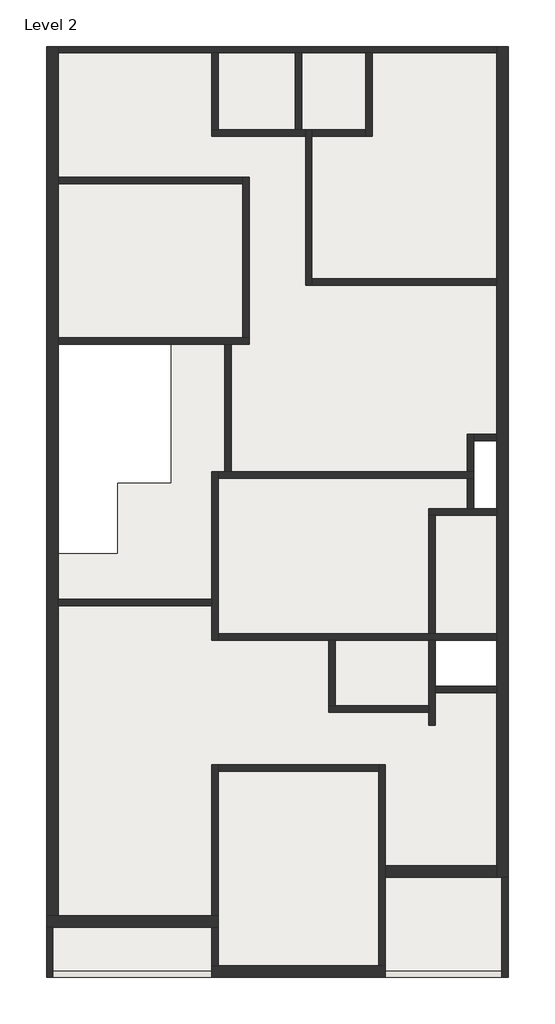
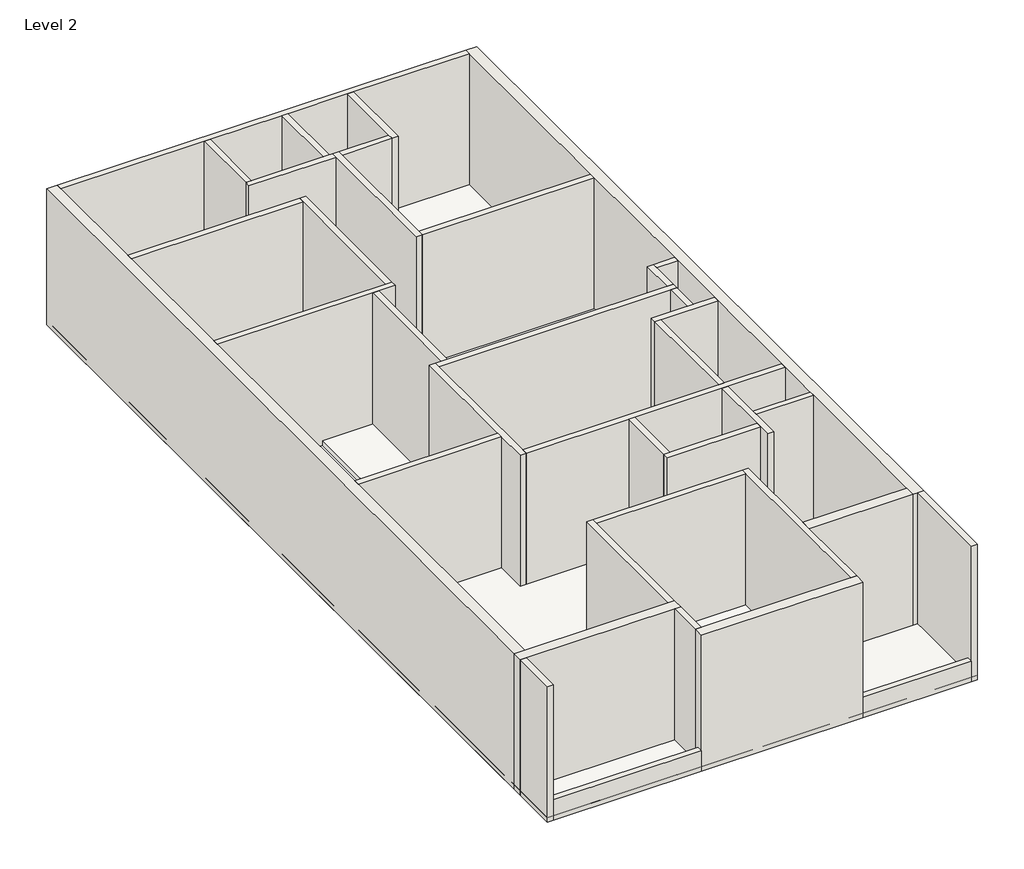
# One storey: 38 walls, 1 roof.
"""IFC4 building model written with IfcOpenShell, lengths in millimetres."""

from ifc_helpers import new_model, si_unit, frame, origin, place, context, project, spatial, polyline, outline, extrude, faceted_brep, element, save

model = new_model("IFC4")

# Units and contexts
model_context = context("Model", 3, world=origin())
ifc_project = project(units=[si_unit("LENGTHUNIT", "METRE", prefix="MILLI")], contexts=[model_context])

# Site, building, storey
site = spatial("IfcSite", under=ifc_project)
building = spatial("IfcBuilding", under=site)
storey = spatial("IfcBuildingStorey", under=building, Name="Level 2", Elevation=3048.0)

# Roof
placement = place(None, origin())
element("IfcRoof", 1, ObjectType="Generic - 12\"", at=placement, inside=storey, context=model_context, shape_type="SweptSolid", body=[
    extrude(outline(polyline([(-6481.5338869, 11814.9468856), (2662.4661131, 11814.9468856), (2662.4661131, -6625.4531144), (-6481.5338869, -6625.4531144), (-6481.5338869, 5922.1468856), (-6481.5338869, 11814.9468856)]), holes=[polyline([(-5084.5338869, 3178.9468856), (-4017.7338869, 3178.9468856), (-4017.7338869, 5922.1468856), (-6252.9338869, 5922.1468856), (-6252.9338869, 1781.9468856), (-5084.5338869, 1781.9468856), (-5084.5338869, 3178.9468856)]), polyline([(2433.8661131, 2658.2468856), (2433.8661131, 4004.4468856), (1976.6661131, 4004.4468856), (1976.6661131, 2658.2468856), (2433.8661131, 2658.2468856)]), polyline([(2433.8661131, -859.6531144), (2433.8661131, 54.7468856), (1214.6661131, 54.7468856), (1214.6661131, -859.6531144), (2433.8661131, -859.6531144)])]), frame((0.0, 0.0, 3048.0), z_axis=(0.0, 0.0, 1.0), x_axis=(1.0, 0.0, 0.0)), (0.0, 0.0, 1.0), 101.6),
])

# Walls
element("IfcWall", 2, ObjectType="Generic - 5\"", at=placement, inside=storey, context=model_context, shape_type="Brep", body=[
    faceted_brep([(-6252.9338869, 5922.1468856, 3048.0), (-2950.9338869, 5922.1468856, 3048.0), (-2823.9338869, 5922.1468856, 3048.0), (-2468.3338869, 5922.1468856, 3048.0), (-2468.3338869, 5922.1468856, 6096.0), (-2823.9338869, 5922.1468856, 6096.0), (-2950.9338869, 5922.1468856, 6096.0), (-6252.9338869, 5922.1468856, 6096.0), (-6252.9338869, 6049.1468856, 3048.0), (-6252.9338869, 6049.1468856, 6096.0), (-2595.3338869, 6049.1468856, 6096.0), (-2468.3338869, 6049.1468856, 6096.0), (-2468.3338869, 6049.1468856, 3048.0), (-2595.3338869, 6049.1468856, 3048.0)], [[[0, 1, 2, 3, 4, 5, 6, 7]], [[8, 9, 10, 11, 12, 13]], [[3, 2, 1, 0, 8, 13, 12]], [[7, 6, 5, 4, 11, 10, 9]], [[4, 3, 12, 11]], [[0, 7, 9, 8]]]),
])
element("IfcWall", 3, ObjectType="Generic - 5\"", at=placement, inside=storey, context=model_context, shape_type="Brep", body=[
    faceted_brep([(-3204.9338869, 3394.8468856, 3048.0), (-3204.9338869, 867.5468856, 3048.0), (-3204.9338869, 740.5468856, 3048.0), (-3204.9338869, 54.7468856, 3048.0), (-3204.9338869, 54.7468856, 6096.0), (-3204.9338869, 740.5468856, 6096.0), (-3204.9338869, 867.5468856, 6096.0), (-3204.9338869, 3394.8468856, 6096.0), (-3077.9338869, 3394.8468856, 3048.0), (-3077.9338869, 3394.8468856, 6096.0), (-3077.9338869, 3267.8468856, 6096.0), (-3077.9338869, 181.7468856, 6096.0), (-3077.9338869, 54.7468856, 6096.0), (-3077.9338869, 54.7468856, 3048.0), (-3077.9338869, 181.7468856, 3048.0), (-3077.9338869, 3267.8468856, 3048.0)], [[[0, 1, 2, 3, 4, 5, 6, 7]], [[8, 9, 10, 11, 12, 13, 14, 15]], [[3, 2, 1, 0, 8, 15, 14, 13]], [[7, 6, 5, 4, 12, 11, 10, 9]], [[4, 3, 13, 12]], [[0, 7, 9, 8]]]),
])
element("IfcWall", 4, ObjectType="Generic - 5\"", at=placement, inside=storey, context=model_context, shape_type="SweptSolid", body=[
    extrude(outline(polyline([(-6252.9338869, 867.5468856), (-3204.9338869, 867.5468856), (-3204.9338869, 740.5468856), (-6252.9338869, 740.5468856), (-6252.9338869, 867.5468856)])), frame((0.0, 0.0, 3048.0), z_axis=(0.0, 0.0, 1.0), x_axis=(1.0, 0.0, 0.0)), (0.0, 0.0, 1.0), 3048.0),
])
element("IfcWall", 5, ObjectType="Generic - 5\"", at=placement, inside=storey, context=model_context, shape_type="Brep", body=[
    faceted_brep([(-3077.9338869, 3267.8468856, 3048.0), (1849.6661131, 3267.8468856, 3048.0), (1976.6661131, 3267.8468856, 3048.0), (1976.6661131, 3267.8468856, 6096.0), (1849.6661131, 3267.8468856, 6096.0), (-3077.9338869, 3267.8468856, 6096.0), (-3077.9338869, 3394.8468856, 3048.0), (-3077.9338869, 3394.8468856, 6096.0), (-2950.9338869, 3394.8468856, 6096.0), (-2823.9338869, 3394.8468856, 6096.0), (1849.6661131, 3394.8468856, 6096.0), (1976.6661131, 3394.8468856, 6096.0), (1976.6661131, 3394.8468856, 3048.0), (1849.6661131, 3394.8468856, 3048.0), (-2823.9338869, 3394.8468856, 3048.0), (-2950.9338869, 3394.8468856, 3048.0)], [[[0, 1, 2, 3, 4, 5]], [[6, 7, 8, 9, 10, 11, 12, 13, 14, 15]], [[2, 1, 0, 6, 15, 14, 13, 12]], [[5, 4, 3, 11, 10, 9, 8, 7]], [[3, 2, 12, 11]], [[0, 5, 7, 6]]]),
])
element("IfcWall", 6, ObjectType="Generic - 5\"", at=placement, inside=storey, context=model_context, shape_type="Brep", body=[
    faceted_brep([(-2468.3338869, 6049.1468856, 3048.0), (-2468.3338869, 9224.1468856, 3048.0), (-2468.3338869, 9224.1468856, 6096.0), (-2468.3338869, 6049.1468856, 6096.0), (-2595.3338869, 6049.1468856, 3048.0), (-2595.3338869, 6049.1468856, 6096.0), (-2595.3338869, 9097.1468856, 6096.0), (-2595.3338869, 9224.1468856, 6096.0), (-2595.3338869, 9224.1468856, 3048.0), (-2595.3338869, 9097.1468856, 3048.0)], [[[0, 1, 2, 3]], [[4, 5, 6, 7, 8, 9]], [[1, 0, 4, 9, 8]], [[3, 2, 7, 6, 5]], [[0, 3, 5, 4]], [[2, 1, 8, 7]]]),
])
element("IfcWall", 7, ObjectType="Generic - 5\"", at=placement, inside=storey, context=model_context, shape_type="SweptSolid", body=[
    extrude(outline(polyline([(-6252.9338869, 9224.1468856), (-2595.3338869, 9224.1468856), (-2595.3338869, 9097.1468856), (-6252.9338869, 9097.1468856), (-6252.9338869, 9224.1468856)])), frame((0.0, 0.0, 3048.0), z_axis=(0.0, 0.0, 1.0), x_axis=(1.0, 0.0, 0.0)), (0.0, 0.0, 1.0), 3048.0),
])
element("IfcWall", 8, ObjectType="Generic - 5\"", at=placement, inside=storey, context=model_context, shape_type="Brep", body=[
    faceted_brep([(-6252.9338869, 11687.9468856, 3048.0), (-3204.9338869, 11687.9468856, 3048.0), (-3077.9338869, 11687.9468856, 3048.0), (-1553.9338869, 11687.9468856, 3048.0), (-1426.9338869, 11687.9468856, 3048.0), (-156.9338869, 11687.9468856, 3048.0), (-29.9338869, 11687.9468856, 3048.0), (2433.8661131, 11687.9468856, 3048.0), (2433.8661131, 11687.9468856, 6096.0), (-29.9338869, 11687.9468856, 6096.0), (-156.9338869, 11687.9468856, 6096.0), (-1426.9338869, 11687.9468856, 6096.0), (-1553.9338869, 11687.9468856, 6096.0), (-3077.9338869, 11687.9468856, 6096.0), (-3204.9338869, 11687.9468856, 6096.0), (-6252.9338869, 11687.9468856, 6096.0), (-6252.9338869, 11814.9468856, 3048.0), (-6252.9338869, 11814.9468856, 6096.0), (2433.8661131, 11814.9468856, 6096.0), (2433.8661131, 11814.9468856, 3048.0)], [[[0, 1, 2, 3, 4, 5, 6, 7, 8, 9, 10, 11, 12, 13, 14, 15]], [[16, 17, 18, 19]], [[7, 6, 5, 4, 3, 2, 1, 0, 16, 19]], [[15, 14, 13, 12, 11, 10, 9, 8, 18, 17]], [[8, 7, 19, 18]], [[0, 15, 17, 16]]]),
])
element("IfcWall", 9, ObjectType="Generic - 5\"", at=placement, inside=storey, context=model_context, shape_type="Brep", body=[
    faceted_brep([(-1350.7338869, 10163.9468856, 3048.0), (-1350.7338869, 10036.9468856, 3048.0), (-1350.7338869, 7090.5468856, 3048.0), (-1350.7338869, 7090.5468856, 6096.0), (-1350.7338869, 10036.9468856, 6096.0), (-1350.7338869, 10163.9468856, 6096.0), (-1223.7338869, 10163.9468856, 3048.0), (-1223.7338869, 10163.9468856, 6096.0), (-1223.7338869, 10036.9468856, 6096.0), (-1223.7338869, 7217.5468856, 6096.0), (-1223.7338869, 7090.5468856, 6096.0), (-1223.7338869, 7090.5468856, 3048.0), (-1223.7338869, 7217.5468856, 3048.0), (-1223.7338869, 10036.9468856, 3048.0)], [[[0, 1, 2, 3, 4, 5]], [[6, 7, 8, 9, 10, 11, 12, 13]], [[2, 1, 0, 6, 13, 12, 11]], [[5, 4, 3, 10, 9, 8, 7]], [[3, 2, 11, 10]], [[0, 5, 7, 6]]]),
])
element("IfcWall", 10, ObjectType="Generic - 5\"", at=placement, inside=storey, context=model_context, shape_type="SweptSolid", body=[
    extrude(outline(polyline([(2433.8661131, 7090.5468856), (-1223.7338869, 7090.5468856), (-1223.7338869, 7217.5468856), (2433.8661131, 7217.5468856), (2433.8661131, 7090.5468856)])), frame((0.0, 0.0, 3048.0), z_axis=(0.0, 0.0, 1.0), x_axis=(1.0, 0.0, 0.0)), (0.0, 0.0, 1.0), 3048.0),
])
element("IfcWall", 11, ObjectType="Generic - 5\"", at=placement, inside=storey, context=model_context, shape_type="Brep", body=[
    faceted_brep([(-3204.9338869, 10036.9468856, 3048.0), (-1350.7338869, 10036.9468856, 3048.0), (-1350.7338869, 10036.9468856, 6096.0), (-3204.9338869, 10036.9468856, 6096.0), (-3204.9338869, 10163.9468856, 3048.0), (-3204.9338869, 10163.9468856, 6096.0), (-3077.9338869, 10163.9468856, 6096.0), (-1553.9338869, 10163.9468856, 6096.0), (-1426.9338869, 10163.9468856, 6096.0), (-1350.7338869, 10163.9468856, 6096.0), (-1350.7338869, 10163.9468856, 3048.0), (-1426.9338869, 10163.9468856, 3048.0), (-1553.9338869, 10163.9468856, 3048.0), (-3077.9338869, 10163.9468856, 3048.0)], [[[0, 1, 2, 3]], [[4, 5, 6, 7, 8, 9, 10, 11, 12, 13]], [[1, 0, 4, 13, 12, 11, 10]], [[3, 2, 9, 8, 7, 6, 5]], [[2, 1, 10, 9]], [[0, 3, 5, 4]]]),
])
element("IfcWall", 12, ObjectType="Generic - 5\"", at=placement, inside=storey, context=model_context, shape_type="SweptSolid", body=[
    extrude(outline(polyline([(-3204.9338869, 10163.9468856), (-3204.9338869, 11687.9468856), (-3077.9338869, 11687.9468856), (-3077.9338869, 10163.9468856), (-3204.9338869, 10163.9468856)])), frame((0.0, 0.0, 3048.0), z_axis=(0.0, 0.0, 1.0), x_axis=(1.0, 0.0, 0.0)), (0.0, 0.0, 1.0), 3048.0),
])
element("IfcWall", 13, ObjectType="Generic - 5\"", at=placement, inside=storey, context=model_context, shape_type="SweptSolid", body=[
    extrude(outline(polyline([(-1553.9338869, 10163.9468856), (-1553.9338869, 11687.9468856), (-1426.9338869, 11687.9468856), (-1426.9338869, 10163.9468856), (-1553.9338869, 10163.9468856)])), frame((0.0, 0.0, 3048.0), z_axis=(0.0, 0.0, 1.0), x_axis=(1.0, 0.0, 0.0)), (0.0, 0.0, 1.0), 3048.0),
])
element("IfcWall", 14, ObjectType="Generic - 5\"", at=placement, inside=storey, context=model_context, shape_type="Brep", body=[
    faceted_brep([(-156.9338869, 11687.9468856, 3048.0), (-156.9338869, 10163.9468856, 3048.0), (-156.9338869, 10036.9468856, 3048.0), (-156.9338869, 10036.9468856, 6096.0), (-156.9338869, 10163.9468856, 6096.0), (-156.9338869, 11687.9468856, 6096.0), (-29.9338869, 11687.9468856, 3048.0), (-29.9338869, 11687.9468856, 6096.0), (-29.9338869, 10036.9468856, 6096.0), (-29.9338869, 10036.9468856, 3048.0)], [[[0, 1, 2, 3, 4, 5]], [[6, 7, 8, 9]], [[2, 1, 0, 6, 9]], [[5, 4, 3, 8, 7]], [[0, 5, 7, 6]], [[3, 2, 9, 8]]]),
])
element("IfcWall", 15, ObjectType="Generic - 5\"", at=placement, inside=storey, context=model_context, shape_type="SweptSolid", body=[
    extrude(outline(polyline([(-1223.7338869, 10163.9468856), (-156.9338869, 10163.9468856), (-156.9338869, 10036.9468856), (-1223.7338869, 10036.9468856), (-1223.7338869, 10163.9468856)])), frame((0.0, 0.0, 3048.0), z_axis=(0.0, 0.0, 1.0), x_axis=(1.0, 0.0, 0.0)), (0.0, 0.0, 1.0), 3048.0),
])
element("IfcWall", 16, ObjectType="Generic - 5\"", at=placement, inside=storey, context=model_context, shape_type="Brep", body=[
    faceted_brep([(2433.8661131, 181.7468856, 3048.0), (1214.6661131, 181.7468856, 3048.0), (1087.6661131, 181.7468856, 3048.0), (-3077.9338869, 181.7468856, 3048.0), (-3077.9338869, 181.7468856, 6096.0), (1087.6661131, 181.7468856, 6096.0), (1214.6661131, 181.7468856, 6096.0), (2433.8661131, 181.7468856, 6096.0), (2433.8661131, 54.7468856, 3048.0), (2433.8661131, 54.7468856, 6096.0), (1214.6661131, 54.7468856, 6096.0), (1087.6661131, 54.7468856, 6096.0), (-766.5338869, 54.7468856, 6096.0), (-893.5338869, 54.7468856, 6096.0), (-3077.9338869, 54.7468856, 6096.0), (-3077.9338869, 54.7468856, 3048.0), (-893.5338869, 54.7468856, 3048.0), (-766.5338869, 54.7468856, 3048.0), (1087.6661131, 54.7468856, 3048.0), (1214.6661131, 54.7468856, 3048.0)], [[[0, 1, 2, 3, 4, 5, 6, 7]], [[8, 9, 10, 11, 12, 13, 14, 15, 16, 17, 18, 19]], [[3, 2, 1, 0, 8, 19, 18, 17, 16, 15]], [[7, 6, 5, 4, 14, 13, 12, 11, 10, 9]], [[0, 7, 9, 8]], [[4, 3, 15, 14]]]),
])
element("IfcWall", 17, ObjectType="Generic - 5\"", at=placement, inside=storey, context=model_context, shape_type="Brep", body=[
    faceted_brep([(1087.6661131, 54.7468856, 3048.0), (1087.6661131, -1240.6531144, 3048.0), (1087.6661131, -1367.6531144, 3048.0), (1087.6661131, -1634.3531144, 3048.0), (1087.6661131, -1634.3531144, 6096.0), (1087.6661131, -1367.6531144, 6096.0), (1087.6661131, -1240.6531144, 6096.0), (1087.6661131, 54.7468856, 6096.0), (1214.6661131, 54.7468856, 3048.0), (1214.6661131, 54.7468856, 6096.0), (1214.6661131, -859.6531144, 6096.0), (1214.6661131, -986.6531144, 6096.0), (1214.6661131, -1634.3531144, 6096.0), (1214.6661131, -1634.3531144, 3048.0), (1214.6661131, -986.6531144, 3048.0), (1214.6661131, -859.6531144, 3048.0)], [[[0, 1, 2, 3, 4, 5, 6, 7]], [[8, 9, 10, 11, 12, 13, 14, 15]], [[3, 2, 1, 0, 8, 15, 14, 13]], [[4, 3, 13, 12]], [[7, 6, 5, 4, 12, 11, 10, 9]], [[0, 7, 9, 8]]]),
])
element("IfcWall", 18, ObjectType="Generic - 5\"", at=placement, inside=storey, context=model_context, shape_type="SweptSolid", body=[
    extrude(outline(polyline([(2433.8661131, -986.6531144), (1214.6661131, -986.6531144), (1214.6661131, -859.6531144), (2433.8661131, -859.6531144), (2433.8661131, -986.6531144)])), frame((0.0, 0.0, 3048.0), z_axis=(0.0, 0.0, 1.0), x_axis=(1.0, 0.0, 0.0)), (0.0, 0.0, 1.0), 3048.0),
])
element("IfcWall", 19, ObjectType="Generic - 5\"", at=placement, inside=storey, context=model_context, shape_type="Brep", body=[
    faceted_brep([(-3077.9338869, -5406.2531144, 3048.0), (-3077.9338869, -2536.0531144, 3048.0), (-3077.9338869, -2409.0531144, 3048.0), (-3077.9338869, -2409.0531144, 6096.0), (-3077.9338869, -2536.0531144, 6096.0), (-3077.9338869, -5406.2531144, 6096.0), (-3204.9338869, -5406.2531144, 3048.0), (-3204.9338869, -5406.2531144, 6096.0), (-3204.9338869, -2409.0531144, 6096.0), (-3204.9338869, -2409.0531144, 3048.0)], [[[0, 1, 2, 3, 4, 5]], [[6, 7, 8, 9]], [[2, 1, 0, 6, 9]], [[5, 4, 3, 8, 7]], [[0, 5, 7, 6]], [[3, 2, 9, 8]]]),
])
element("IfcWall", 20, ObjectType="Generic - 5\"", at=placement, inside=storey, context=model_context, shape_type="Brep", body=[
    faceted_brep([(1976.6661131, 3394.8468856, 3048.0), (1976.6661131, 4004.4468856, 3048.0), (1976.6661131, 4131.4468856, 3048.0), (1976.6661131, 4131.4468856, 6096.0), (1976.6661131, 4004.4468856, 6096.0), (1976.6661131, 3394.8468856, 6096.0), (1849.6661131, 3394.8468856, 3048.0), (1849.6661131, 3394.8468856, 6096.0), (1849.6661131, 4131.4468856, 6096.0), (1849.6661131, 4131.4468856, 3048.0)], [[[0, 1, 2, 3, 4, 5]], [[6, 7, 8, 9]], [[2, 1, 0, 6, 9]], [[5, 4, 3, 8, 7]], [[0, 5, 7, 6]], [[3, 2, 9, 8]]]),
])
element("IfcWall", 21, ObjectType="Generic - 5\"", at=placement, inside=storey, context=model_context, shape_type="SweptSolid", body=[
    extrude(outline(polyline([(2433.8661131, 4004.4468856), (1976.6661131, 4004.4468856), (1976.6661131, 4131.4468856), (2433.8661131, 4131.4468856), (2433.8661131, 4004.4468856)])), frame((0.0, 0.0, 3048.0), z_axis=(0.0, 0.0, 1.0), x_axis=(1.0, 0.0, 0.0)), (0.0, 0.0, 1.0), 3048.0),
])
element("IfcWall", 22, ObjectType="Generic - 5\"", at=placement, inside=storey, context=model_context, shape_type="SweptSolid", body=[
    extrude(outline(polyline([(1849.6661131, 2658.2468856), (1849.6661131, 3267.8468856), (1976.6661131, 3267.8468856), (1976.6661131, 2658.2468856), (1849.6661131, 2658.2468856)])), frame((0.0, 0.0, 3048.0), z_axis=(0.0, 0.0, 1.0), x_axis=(1.0, 0.0, 0.0)), (0.0, 0.0, 1.0), 3048.0),
])
element("IfcWall", 23, ObjectType="Generic - 5\"", at=placement, inside=storey, context=model_context, shape_type="Brep", body=[
    faceted_brep([(1087.6661131, 2531.2468856, 3048.0), (1214.6661131, 2531.2468856, 3048.0), (2433.8661131, 2531.2468856, 3048.0), (2433.8661131, 2531.2468856, 6096.0), (1214.6661131, 2531.2468856, 6096.0), (1087.6661131, 2531.2468856, 6096.0), (1087.6661131, 2658.2468856, 3048.0), (1087.6661131, 2658.2468856, 6096.0), (1849.6661131, 2658.2468856, 6096.0), (1976.6661131, 2658.2468856, 6096.0), (2433.8661131, 2658.2468856, 6096.0), (2433.8661131, 2658.2468856, 3048.0), (1976.6661131, 2658.2468856, 3048.0), (1849.6661131, 2658.2468856, 3048.0)], [[[0, 1, 2, 3, 4, 5]], [[6, 7, 8, 9, 10, 11, 12, 13]], [[2, 1, 0, 6, 13, 12, 11]], [[5, 4, 3, 10, 9, 8, 7]], [[3, 2, 11, 10]], [[0, 5, 7, 6]]]),
])
element("IfcWall", 24, ObjectType="Generic - 5\"", at=placement, inside=storey, context=model_context, shape_type="SweptSolid", body=[
    extrude(outline(polyline([(1214.6661131, 2531.2468856), (1214.6661131, 181.7468856), (1087.6661131, 181.7468856), (1087.6661131, 2531.2468856), (1214.6661131, 2531.2468856)])), frame((0.0, 0.0, 3048.0), z_axis=(0.0, 0.0, 1.0), x_axis=(1.0, 0.0, 0.0)), (0.0, 0.0, 1.0), 3048.0),
])
element("IfcWall", 25, ObjectType="Generic - 5\"", at=placement, inside=storey, context=model_context, shape_type="Brep", body=[
    faceted_brep([(1087.6661131, -1240.6531144, 3048.0), (-766.5338869, -1240.6531144, 3048.0), (-893.5338869, -1240.6531144, 3048.0), (-893.5338869, -1240.6531144, 6096.0), (-766.5338869, -1240.6531144, 6096.0), (1087.6661131, -1240.6531144, 6096.0), (1087.6661131, -1367.6531144, 3048.0), (1087.6661131, -1367.6531144, 6096.0), (-893.5338869, -1367.6531144, 6096.0), (-893.5338869, -1367.6531144, 3048.0)], [[[0, 1, 2, 3, 4, 5]], [[6, 7, 8, 9]], [[2, 1, 0, 6, 9]], [[5, 4, 3, 8, 7]], [[3, 2, 9, 8]], [[0, 5, 7, 6]]]),
])
element("IfcWall", 26, ObjectType="Generic - 5\"", at=placement, inside=storey, context=model_context, shape_type="SweptSolid", body=[
    extrude(outline(polyline([(-766.5338869, 54.7468856), (-766.5338869, -1240.6531144), (-893.5338869, -1240.6531144), (-893.5338869, 54.7468856), (-766.5338869, 54.7468856)])), frame((0.0, 0.0, 3048.0), z_axis=(0.0, 0.0, 1.0), x_axis=(1.0, 0.0, 0.0)), (0.0, 0.0, 1.0), 3048.0),
])
element("IfcWall", 27, ObjectType="Generic - 5\"", at=placement, inside=storey, context=model_context, shape_type="Brep", body=[
    faceted_brep([(97.0661131, -2409.0531144, 3048.0), (97.0661131, -2536.0531144, 3048.0), (97.0661131, -6396.8531144, 3048.0), (97.0661131, -6396.8531144, 6096.0), (97.0661131, -2536.0531144, 6096.0), (97.0661131, -2409.0531144, 6096.0), (224.0661131, -2409.0531144, 3048.0), (224.0661131, -2409.0531144, 6096.0), (224.0661131, -4415.6531144, 6096.0), (224.0661131, -4644.2531144, 6096.0), (224.0661131, -6396.8531144, 6096.0), (224.0661131, -6396.8531144, 3048.0), (224.0661131, -4644.2531144, 3048.0), (224.0661131, -4415.6531144, 3048.0)], [[[0, 1, 2, 3, 4, 5]], [[6, 7, 8, 9, 10, 11, 12, 13]], [[2, 1, 0, 6, 13, 12, 11]], [[5, 4, 3, 10, 9, 8, 7]], [[0, 5, 7, 6]], [[2, 11, 10, 3]]]),
])
element("IfcWall", 28, ObjectType="Generic - 5\"", at=placement, inside=storey, context=model_context, shape_type="Brep", body=[
    faceted_brep([(-6481.5338869, -5634.8531144, 3048.0), (-6481.5338869, -6625.4531144, 3048.0), (-6481.5338869, -6625.4531144, 6096.0), (-6481.5338869, -5634.8531144, 6096.0), (-6354.5338869, -5634.8531144, 3048.0), (-6354.5338869, -5634.8531144, 6096.0), (-6354.5338869, -6625.4531144, 6096.0), (-6354.5338869, -6625.4531144, 3505.2), (-6354.5338869, -6625.4531144, 3048.0), (-6354.5338869, -6498.4531144, 3048.0)], [[[0, 1, 2, 3]], [[4, 5, 6, 7, 8, 9]], [[1, 0, 4, 9, 8]], [[3, 2, 6, 5]], [[0, 3, 5, 4]], [[2, 1, 8, 7, 6]]]),
])
element("IfcWall", 29, ObjectType="Generic - 5\"", at=placement, inside=storey, context=model_context, shape_type="SweptSolid", body=[
    extrude(outline(polyline([(-3204.9338869, -6625.4531144), (-6354.5338869, -6625.4531144), (-6354.5338869, -6498.4531144), (-3204.9338869, -6498.4531144), (-3204.9338869, -6625.4531144)])), frame((0.0, 0.0, 3048.0), z_axis=(0.0, 0.0, 1.0), x_axis=(1.0, 0.0, 0.0)), (0.0, 0.0, 1.0), 457.2),
])
element("IfcWall", 30, ObjectType="Generic - 5\"", at=placement, inside=storey, context=model_context, shape_type="Brep", body=[
    faceted_brep([(2662.4661131, -6625.4531144, 3048.0), (2662.4661131, -4644.2531144, 3048.0), (2662.4661131, -4644.2531144, 6096.0), (2662.4661131, -6625.4531144, 6096.0), (2535.4661131, -6625.4531144, 3048.0), (2535.4661131, -6625.4531144, 3505.2), (2535.4661131, -6625.4531144, 6096.0), (2535.4661131, -4644.2531144, 6096.0), (2535.4661131, -4644.2531144, 3048.0), (2535.4661131, -6498.4531144, 3048.0)], [[[0, 1, 2, 3]], [[4, 5, 6, 7, 8, 9]], [[1, 0, 4, 9, 8]], [[3, 2, 7, 6]], [[2, 1, 8, 7]], [[0, 3, 6, 5, 4]]]),
])
element("IfcWall", 31, ObjectType="Generic - 5\"", at=placement, inside=storey, context=model_context, shape_type="SweptSolid", body=[
    extrude(outline(polyline([(-3204.9338869, -6396.8531144), (-3204.9338869, -5634.8531144), (-3077.9338869, -5634.8531144), (-3077.9338869, -6396.8531144), (-3204.9338869, -6396.8531144)])), frame((0.0, 0.0, 3048.0), z_axis=(0.0, 0.0, 1.0), x_axis=(1.0, 0.0, 0.0)), (0.0, 0.0, 1.0), 3048.0),
])
element("IfcWall", 32, ObjectType="Generic - 5\"", at=placement, inside=storey, context=model_context, shape_type="SweptSolid", body=[
    extrude(outline(polyline([(2535.4661131, -6625.4531144), (224.0661131, -6625.4531144), (224.0661131, -6498.4531144), (2535.4661131, -6498.4531144), (2535.4661131, -6625.4531144)])), frame((0.0, 0.0, 3048.0), z_axis=(0.0, 0.0, 1.0), x_axis=(1.0, 0.0, 0.0)), (0.0, 0.0, 1.0), 457.2),
])
element("IfcWall", 33, ObjectType="Generic - 5\"", at=placement, inside=storey, context=model_context, shape_type="SweptSolid", body=[
    extrude(outline(polyline([(97.0661131, -2536.0531144), (-3077.9338869, -2536.0531144), (-3077.9338869, -2409.0531144), (97.0661131, -2409.0531144), (97.0661131, -2536.0531144)])), frame((0.0, 0.0, 3048.0), z_axis=(0.0, 0.0, 1.0), x_axis=(1.0, 0.0, 0.0)), (0.0, 0.0, 1.0), 3048.0),
])
element("IfcWall", 34, ObjectType="Generic - 5\"", at=placement, inside=storey, context=model_context, shape_type="SweptSolid", body=[
    extrude(outline(polyline([(-2950.9338869, 3394.8468856), (-2950.9338869, 5922.1468856), (-2823.9338869, 5922.1468856), (-2823.9338869, 3394.8468856), (-2950.9338869, 3394.8468856)])), frame((0.0, 0.0, 3048.0), z_axis=(0.0, 0.0, 1.0), x_axis=(1.0, 0.0, 0.0)), (0.0, 0.0, 1.0), 3048.0),
])
element("IfcWall", 35, ObjectType="Generic - 9\"", at=placement, inside=storey, context=model_context, shape_type="Brep", body=[
    faceted_brep([(2433.8661131, 11814.9468856, 3048.0), (2433.8661131, 11687.9468856, 3048.0), (2433.8661131, 7217.5468856, 3048.0), (2433.8661131, 7090.5468856, 3048.0), (2433.8661131, 4131.4468856, 3048.0), (2433.8661131, 4004.4468856, 3048.0), (2433.8661131, 2658.2468856, 3048.0), (2433.8661131, 2531.2468856, 3048.0), (2433.8661131, 181.7468856, 3048.0), (2433.8661131, 54.7468856, 3048.0), (2433.8661131, -859.6531144, 3048.0), (2433.8661131, -986.6531144, 3048.0), (2433.8661131, -4415.6531144, 3048.0), (2433.8661131, -4644.2531144, 3048.0), (2433.8661131, -4644.2531144, 6096.0), (2433.8661131, -4415.6531144, 6096.0), (2433.8661131, -986.6531144, 6096.0), (2433.8661131, -859.6531144, 6096.0), (2433.8661131, 54.7468856, 6096.0), (2433.8661131, 181.7468856, 6096.0), (2433.8661131, 2531.2468856, 6096.0), (2433.8661131, 2658.2468856, 6096.0), (2433.8661131, 4004.4468856, 6096.0), (2433.8661131, 4131.4468856, 6096.0), (2433.8661131, 7090.5468856, 6096.0), (2433.8661131, 7217.5468856, 6096.0), (2433.8661131, 11687.9468856, 6096.0), (2433.8661131, 11814.9468856, 6096.0), (2662.4661131, 11814.9468856, 3048.0), (2662.4661131, 11814.9468856, 6096.0), (2662.4661131, -4644.2531144, 6096.0), (2662.4661131, -4644.2531144, 3048.0), (2535.4661131, -4644.2531144, 3048.0), (2535.4661131, -4644.2531144, 6096.0)], [[[0, 1, 2, 3, 4, 5, 6, 7, 8, 9, 10, 11, 12, 13, 14, 15, 16, 17, 18, 19, 20, 21, 22, 23, 24, 25, 26, 27]], [[28, 29, 30, 31]], [[13, 12, 11, 10, 9, 8, 7, 6, 5, 4, 3, 2, 1, 0, 28, 31, 32]], [[27, 26, 25, 24, 23, 22, 21, 20, 19, 18, 17, 16, 15, 14, 33, 30, 29]], [[0, 27, 29, 28]], [[14, 13, 32, 31, 30, 33]]]),
])
element("IfcWall", 36, ObjectType="Generic - 9\"", at=placement, inside=storey, context=model_context, shape_type="Brep", body=[
    faceted_brep([(-6252.9338869, -5406.2531144, 3048.0), (-6252.9338869, 740.5468856, 3048.0), (-6252.9338869, 867.5468856, 3048.0), (-6252.9338869, 5922.1468856, 3048.0), (-6252.9338869, 6049.1468856, 3048.0), (-6252.9338869, 9097.1468856, 3048.0), (-6252.9338869, 9224.1468856, 3048.0), (-6252.9338869, 11687.9468856, 3048.0), (-6252.9338869, 11814.9468856, 3048.0), (-6252.9338869, 11814.9468856, 6096.0), (-6252.9338869, 11687.9468856, 6096.0), (-6252.9338869, 9224.1468856, 6096.0), (-6252.9338869, 9097.1468856, 6096.0), (-6252.9338869, 6049.1468856, 6096.0), (-6252.9338869, 5922.1468856, 6096.0), (-6252.9338869, 867.5468856, 6096.0), (-6252.9338869, 740.5468856, 6096.0), (-6252.9338869, -5406.2531144, 6096.0), (-6481.5338869, -5406.2531144, 3048.0), (-6481.5338869, -5406.2531144, 6096.0), (-6481.5338869, 11814.9468856, 6096.0), (-6481.5338869, 11814.9468856, 3048.0)], [[[0, 1, 2, 3, 4, 5, 6, 7, 8, 9, 10, 11, 12, 13, 14, 15, 16, 17]], [[18, 19, 20, 21]], [[8, 7, 6, 5, 4, 3, 2, 1, 0, 18, 21]], [[9, 8, 21, 20]], [[17, 16, 15, 14, 13, 12, 11, 10, 9, 20, 19]], [[0, 17, 19, 18]]]),
])
element("IfcWall", 37, ObjectType="Generic - 9\"", at=placement, inside=storey, context=model_context, shape_type="Brep", body=[
    faceted_brep([(-3077.9338869, -5406.2531144, 3048.0), (-3204.9338869, -5406.2531144, 3048.0), (-6252.9338869, -5406.2531144, 3048.0), (-6481.5338869, -5406.2531144, 3048.0), (-6481.5338869, -5406.2531144, 6096.0), (-6252.9338869, -5406.2531144, 6096.0), (-3204.9338869, -5406.2531144, 6096.0), (-3077.9338869, -5406.2531144, 6096.0), (-3077.9338869, -5634.8531144, 3048.0), (-3077.9338869, -5634.8531144, 6096.0), (-3204.9338869, -5634.8531144, 6096.0), (-6354.5338869, -5634.8531144, 6096.0), (-6481.5338869, -5634.8531144, 6096.0), (-6481.5338869, -5634.8531144, 3048.0), (-6354.5338869, -5634.8531144, 3048.0), (-3204.9338869, -5634.8531144, 3048.0)], [[[0, 1, 2, 3, 4, 5, 6, 7]], [[8, 9, 10, 11, 12, 13, 14, 15]], [[3, 2, 1, 0, 8, 15, 14, 13]], [[7, 6, 5, 4, 12, 11, 10, 9]], [[4, 3, 13, 12]], [[0, 7, 9, 8]]]),
])
element("IfcWall", 38, ObjectType="Generic - 9\"", at=placement, inside=storey, context=model_context, shape_type="Brep", body=[
    faceted_brep([(-3204.9338869, -6625.4531144, 6096.0), (-3204.9338869, -6625.4531144, 3505.2), (-3204.9338869, -6625.4531144, 3048.0), (224.0661131, -6625.4531144, 3048.0), (224.0661131, -6625.4531144, 3505.2), (224.0661131, -6625.4531144, 6096.0), (-3204.9338869, -6396.8531144, 3048.0), (-3204.9338869, -6396.8531144, 6096.0), (-3077.9338869, -6396.8531144, 6096.0), (97.0661131, -6396.8531144, 6096.0), (224.0661131, -6396.8531144, 6096.0), (224.0661131, -6396.8531144, 3048.0), (97.0661131, -6396.8531144, 3048.0), (-3077.9338869, -6396.8531144, 3048.0), (-3204.9338869, -6498.4531144, 3048.0), (224.0661131, -6498.4531144, 3048.0)], [[[0, 1, 2, 3, 4, 5]], [[6, 7, 8, 9, 10, 11, 12, 13]], [[3, 2, 14, 6, 13, 12, 11, 15]], [[0, 5, 10, 9, 8, 7]], [[0, 7, 6, 14, 2, 1]], [[3, 15, 11, 10, 5, 4]]]),
])
element("IfcWall", 39, ObjectType="Generic - 9\"", at=placement, inside=storey, context=model_context, shape_type="SweptSolid", body=[
    extrude(outline(polyline([(224.0661131, -4415.6531144), (2433.8661131, -4415.6531144), (2433.8661131, -4644.2531144), (224.0661131, -4644.2531144), (224.0661131, -4415.6531144)])), frame((0.0, 0.0, 3048.0), z_axis=(0.0, 0.0, 1.0), x_axis=(1.0, 0.0, 0.0)), (0.0, 0.0, 1.0), 3048.0),
])

save(model, "model.ifc")

# Revit data of these elements
# Type "Generic - 12\""
#   Assembly Code = "B1020"
#   Layers, outside or top first: 0' - 4" no material (function 1)
# Type "Generic - 5\""
#   Assembly Code = "B2010"
#   Layers, outside or top first: 0' - 5" no material (function 1)
# Type "Generic - 9\""
#   Assembly Code = "B2010"
#   Layers, outside or top first: 0' - 9" no material (function 1)
# Element 1 (IfcRoof, "Generic - 12\"")
#   built-in parameter 1001705 = 10.3333 (stored number, unit not read)
#   built-in parameter 1001710 = 33615
#   Phase Created = New Construction
#   Materials on its faces: "Default Roof"
# Elements 2, 3, 4, 5, 6, 7, 8, 9, 10, 11, 12, 13, 14, 15, 16, 17, 18, 19, 20, 21, 22, 23, 24, 25, 26, 27, 28, 30, 31, 33, 34 (IfcWall, "Generic - 5\"")
#   Top Offset = 0' - 0"
#   Base Offset = 0' - 0"
#   Unconnected Height = 10' - 0"
#   wall height = 10' - 0"
#   Phase Created = New Construction
#   Base Constraint = Level 2
#   Materials on its faces: "Default Wall"
# Elements 29, 32 (IfcWall, "Generic - 5\"")
#   Top Offset = 0' - 0"
#   Base Offset = 0' - 0"
#   Unconnected Height = 1' - 6"
#   wall height = 1' - 6"
#   Phase Created = New Construction
#   Base Constraint = Level 2
#   Materials on its faces: "Default Wall"
# Elements 35, 36, 37, 38, 39 (IfcWall, "Generic - 9\"")
#   Top Offset = 0' - 0"
#   Base Offset = 0' - 0"
#   Unconnected Height = 10' - 0"
#   wall height = 10' - 0"
#   Phase Created = New Construction
#   Base Constraint = Level 2
#   Materials on its faces: "Default Wall"
# Materials
#   "Default Roof": colour RGB 80 80 80, transparency 0
#   "Default Wall": colour RGB 80 80 80, transparency 0
